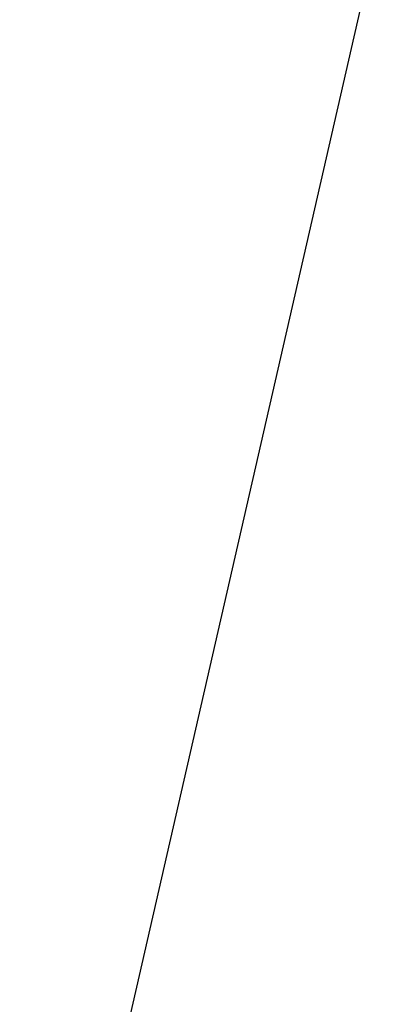
# Model space of a CAD drawing. Units: inches. Extents: x 3590 to 5167, y 65 to 1917.
# Tile 89 of 100: x 5052.4275 to 5052.5773, y 1788.6144 to 1789.0318. Entities that reach past the tile are written whole.
import ezdxf

# ---------------------------------------------------------------- set-up
doc = ezdxf.new("R2010")
doc.units = ezdxf.units.IN
for name, color, linetype, lineweight in [('A-ANNO-DIMS', 2, 'Continuous', 18), ('A-FLOR-PATT', 8, 'Continuous', 13), ('L-PLNT', 94, 'Continuous', 18)]:
    doc.layers.add(name, color=color, linetype=linetype, lineweight=lineweight)
doc.layers.add('DIENHOA', color=3, linetype='Continuous')
doc.styles.get("Standard").update_dxf_attribs({"font": 'arial.ttf'})
doc.dimstyles.new('ISO-25', dxfattribs={"dimtxt": 9, "dimasz": 2.5, "dimexe": 1.25, "dimexo": 0.625, "dimtad": 1, "dimdec": 1, "dimlunit": 3, "dimtxsty": 'Standard', "dimcen": 2.5, "dimadec": 0, "dimazin": 0, "dimtfac": 1, "dimtdec": 1, "dimtmove": 0, "dimatfit": 3, "dimfxl": 1, "dimarcsym": 0})

# ---------------------------------------------------------------- blocks, each defined once
blk = doc.blocks.new('Cay03_mb')
at = {"layer": 'DIENHOA'}
blk.add_lwpolyline([(112.868, 491.948), (95.994, 419.691), (79.461, 347.371), (63.915, 276.46), (50.006, 208.43), (38.381, 144.752), (29.688, 86.901), (24.574, 36.346), (23.687, -5.439)], dxfattribs=at)
blk = doc.blocks.new('*D323')
at = {"layer": 'A-ANNO-DIMS', "color": 0, "lineweight": -2, "transparency": 16777216}
for p, q in [((5069.17227, 1795.21603), (5069.17227, 1874.95034)), ((5065.43703, 1795.21603), (5070.42227, 1795.21603)), ((5069.17227, 1769.30924), (5069.17227, 1792.71603)), ((5065.43703, 1766.80924), (5070.42227, 1766.80924))]:
    blk.add_line(p, q, dxfattribs=at)
at = {"layer": 'A-ANNO-DIMS', "color": 0, "transparency": 16777216}
for points in [[(5068.75561, 1792.71603), (5069.58894, 1792.71603), (5069.17227, 1795.21603)], [(5068.75561, 1769.30924), (5069.58894, 1769.30924), (5069.17227, 1766.80924)]]:
    blk.add_solid(points, dxfattribs=at)
at = {"layer": 'Defpoints', "color": 0, "transparency": 16777216}
for p in [(5064.81203, 1795.21603), (5069.17227, 1795.21603), (5064.81203, 1766.80924)]:
    blk.add_point(p, dxfattribs=at)
at = {"layer": 'A-ANNO-DIMS', "color": 0, "transparency": 16777216, "insert": (5063.89379, 1836.33318), "char_height": 9, "attachment_point": 5, "rotation": 90}
blk.add_mtext('2\'-4 1/2" TYP.', dxfattribs=at)

msp = doc.modelspace()

# ---------------------------------------------------------------- hatches: boundary and pattern name
at = {"layer": 'A-FLOR-PATT', "transparency": 33554687}
h = msp.add_hatch(dxfattribs=at)
h.set_pattern_fill('AR-HBONE', color=256, scale=0.2)
h.set_pattern_definition([(45, (-588.972, 0), (0, 28.73682), [60.96, -20.32]), (135, (-574.604, 14.368), (3e-15, 28.73682), [60.96, -20.32])])
h.paths.add_polyline_path([(5071.27403, 1796.99898), (4933.27403, 1796.99898), (4933.27403, 1753.99898), (4962.77403, 1753.99898, -0.414214), (4928.77403, 1719.99898), (4933.27403, 1718.99898), (4933.27403, 1334.99898), (5071.27403, 1334.99898)])
h.paths.add_polyline_path([(4951.78002, 1521.0767), (4951.7151, 1521.0404), (4951.56345, 1520.89532)], flags=16)
h.paths.add_polyline_path([(4952.267, 1521.37645), (4952.1977, 1521.37111), (4952.19823, 1521.35558)], flags=0)
h.paths.add_polyline_path([(4967.05076, 1529.72832), (4965.23122, 1528.69444), (4963.41109, 1527.71401), (4961.75649, 1526.85081), (4963.58887, 1527.44938), (4964.03555, 1527.47802), (4962.9755, 1527.24902), (4961.76022, 1526.85203), (4959.79219, 1525.83406), (4958.00498, 1524.89483), (4956.24031, 1523.92961), (4954.50395, 1522.91854), (4954.1294, 1522.68163), (4953.36051, 1521.99688), (4953.36558, 1521.99754), (4953.605, 1522.06367), (4955.10605, 1522.76083), (4956.92108, 1523.43405), (4958.67784, 1523.91513), (4960.35834, 1524.20036), (4961.94456, 1524.28606), (4964.17144, 1524.10849), (4965.95752, 1523.30903), (4963.86273, 1522.97565), (4965.18742, 1522.49898), (4963.36614, 1522.49715), (4961.54526, 1522.48682), (4959.76359, 1522.46077), (4958.30414, 1522.4188), (4957.97356, 1522.38829), (4956.30692, 1522.2324), (4954.71821, 1522.07143), (4953.25077, 1521.89915), (4953.52509, 1521.62277), (4954.33087, 1521.37883), (4956.24263, 1521.22987), (4958.03913, 1520.92952), (4959.68424, 1520.48339), (4961.16007, 1519.89569), (4963.10699, 1518.80022), (4964.39286, 1517.32518), (4962.97306, 1517.72596), (4964.55841, 1516.66059), (4965.40664, 1515.70779), (4963.50733, 1516.32179), (4961.67995, 1517.0051), (4959.93478, 1517.74489), (4958.2821, 1518.52833), (4956.73216, 1519.34257), (4955.29527, 1520.17478), (4954.67155, 1520.57237), (4954.51279, 1520.6271), (4955.65848, 1519.31837), (4956.70263, 1517.98232), (4957.64403, 1516.64663), (4958.48545, 1515.33439), (4959.54998, 1513.52398), (4960.43768, 1511.76936), (4958.84107, 1513.6196), (4957.45175, 1515.3249), (4955.8186, 1517.45855), (4956.66537, 1515.44764), (4957.11109, 1513.92292), (4957.44681, 1511.71434), (4957.07641, 1509.79288), (4956.53757, 1511.1103), (4955.99231, 1512.56892), (4955.44448, 1514.12509), (4954.89794, 1515.73518), (4954.35653, 1517.35553), (4953.82412, 1518.94251), (4953.30455, 1520.45247), (4953.06452, 1521.11563), (4952.97143, 1521.14607), (4952.94932, 1521.08646), (4952.72981, 1520.19905), (4953.3698, 1518.02364), (4953.75708, 1516.37279), (4954.05124, 1514.76538), (4954.26449, 1513.22121), (4954.47124, 1511.13121), (4954.4971, 1510.40174), (4954.40903, 1511.76006), (4954.26449, 1513.22121), (4954.05124, 1514.76538), (4953.75708, 1516.37279), (4953.3698, 1518.02364), (4952.87718, 1519.69813), (4952.7161, 1520.1412), (4952.53301, 1519.05871), (4952.37428, 1517.78881), (4952.21925, 1516.31167), (4952.04598, 1514.59986), (4951.83253, 1512.62598), (4951.55697, 1510.36259), (4951.20331, 1512.16818), (4950.85168, 1514.33931), (4950.98529, 1516.37594), (4951.6596, 1518.28625), (4952.59261, 1520.48085), (4952.35664, 1521.1299), (4951.85502, 1520.32753), (4950.83901, 1518.90828), (4949.77675, 1517.58658), (4948.91554, 1516.61731), (4948.11099, 1515.2561), (4947.0891, 1513.55389), (4945.88937, 1511.61495), (4946.32587, 1513.40232), (4946.5624, 1514.24913), (4945.52771, 1513.32668), (4944.58105, 1512.53126), (4946.01774, 1514.50825), (4947.2044, 1516.04763), (4947.89331, 1517.31331), (4949.30686, 1518.76446), (4950.41417, 1519.76716), (4950.45131, 1519.80628), (4952.267, 1521.37645), (4951.64457, 1521.49317), (4950.40371, 1521.17954), (4948.04447, 1520.35868), (4946.11863, 1519.45198), (4944.57182, 1518.47484), (4943.34962, 1517.44265), (4941.99695, 1515.91971), (4941.66146, 1515.27475), (4942.81332, 1516.98973), (4944.57182, 1518.47484), (4946.11863, 1519.45198), (4948.04447, 1520.35868), (4950.40371, 1521.17954), (4951.64457, 1521.49317), (4949.64678, 1521.86781), (4948.59979, 1521.75633), (4947.12629, 1521.5699), (4945.42015, 1521.34763), (4943.44969, 1521.10462), (4941.18319, 1520.85596), (4942.86028, 1521.61265), (4943.87308, 1522.03014), (4942.95216, 1521.9093), (4941.40968, 1521.48512), (4939.54287, 1520.67019), (4938.96775, 1520.2255), (4940.73284, 1521.29899), (4942.95216, 1521.9093), (4943.70184, 1522.00767), (4945.89419, 1522.69998), (4947.56488, 1522.71399), (4948.92086, 1522.56573), (4951.13144, 1522.18271), (4950.97062, 1522.2969), (4948.12924, 1523.00563), (4946.03496, 1523.70671), (4944.23235, 1524.52143), (4942.70692, 1525.46111), (4941.44419, 1526.53707), (4940.42968, 1527.76062), (4939.6489, 1529.14306), (4941.42091, 1528.12232), (4943.14742, 1527.13248), (4944.84093, 1526.17457), (4946.51394, 1525.24959), (4948.17893, 1524.35855), (4948.36457, 1524.26336), (4946.47531, 1526.04459), (4945.18083, 1527.54042), (4944.19039, 1529.03339), (4943.49559, 1530.53985), (4943.27808, 1531.3597), (4942.49849, 1531.91903), (4943.11353, 1531.76249), (4942.95927, 1533.6586), (4944.13953, 1531.9886), (4944.61171, 1531.32339), (4946.20163, 1530.46341), (4947.48567, 1529.50925), (4948.79027, 1528.22649), (4950.36754, 1526.23746), (4949.48547, 1528.15549), (4948.85128, 1530.12254), (4948.49054, 1532.04127), (4948.38105, 1533.91822), (4948.50062, 1535.7599), (4948.82704, 1537.57284), (4949.41803, 1535.56526), (4949.95684, 1533.56932), (4950.46414, 1531.5861), (4950.96058, 1529.6167), (4951.3911, 1527.95448), (4951.72352, 1530.68689), (4952.20106, 1532.57994), (4952.88914, 1534.32964), (4953.77035, 1535.95123), (4954.82726, 1537.45995), (4954.52145, 1535.38966), (4954.27314, 1533.93684), (4955.57999, 1535.6627), (4956.74758, 1536.73859), (4956.15852, 1534.78029), (4955.58917, 1532.87334), (4955.04336, 1531.00581), (4954.52493, 1529.16576), (4954.03771, 1527.34127), (4953.63833, 1525.73298), (4953.61143, 1525.58564), (4953.39805, 1524.16565), (4953.38219, 1524.00887), (4954.06955, 1525.47563), (4954.91212, 1527.02173), (4956.13627, 1528.89351), (4957.84668, 1530.57701), (4959.37601, 1531.54014), (4958.25596, 1530.10398), (4957.14284, 1528.66291), (4956.06626, 1527.24305), (4955.05579, 1525.87054), (4954.14104, 1524.57149), (4953.35159, 1523.37204), (4953.31079, 1523.30299), (4953.27253, 1522.92478), (4953.26102, 1522.38213), (4954.1031, 1523.37273), (4954.63005, 1524.28376), (4955.96149, 1526.35767), (4957.23002, 1528.12969), (4958.42057, 1529.60864), (4960.03671, 1531.36792), (4961.3736, 1532.3752), (4962.1015, 1532.77), (4961.06994, 1531.06113), (4959.98733, 1529.43811), (4958.86851, 1527.90803), (4958.15046, 1527.00742), (4959.80291, 1528.00314), (4961.58854, 1528.79257), (4963.39087, 1529.32783), (4965.21118, 1529.63205)], flags=16)
h.paths.add_polyline_path([(4962.94387, 1523.18187), (4961.10714, 1523.42192), (4960.39205, 1523.36158), (4962.34964, 1523.33061)], flags=0)
h.paths.add_polyline_path([(5049.54129, 1584.55089), (5049.47636, 1584.51458), (5049.32471, 1584.3695)], flags=16)
h.paths.add_polyline_path([(5050.02827, 1584.85063), (5049.95897, 1584.84529), (5049.95949, 1584.82976)], flags=0)
h.paths.add_polyline_path([(5042.33308, 1581.94902), (5043.8799, 1582.92616), (5045.80573, 1583.83286), (5048.16498, 1584.65372), (5049.40583, 1584.96736), (5047.40804, 1585.34199), (5046.36106, 1585.23052), (5044.88755, 1585.04408), (5043.18142, 1584.82181), (5041.21095, 1584.5788), (5038.94446, 1584.33014), (5040.62155, 1585.08683), (5041.63434, 1585.50432), (5040.71343, 1585.38348), (5039.17095, 1584.9593), (5037.30414, 1584.14438), (5036.72901, 1583.69969), (5038.4941, 1584.77317), (5040.71343, 1585.38348), (5041.4631, 1585.48185), (5043.65545, 1586.17416), (5045.32615, 1586.18818), (5046.68212, 1586.03992), (5048.8927, 1585.6569), (5048.73188, 1585.77108), (5045.89051, 1586.47981), (5043.79622, 1587.18089), (5041.99361, 1587.99561), (5040.46818, 1588.9353), (5039.20546, 1590.01125), (5038.19095, 1591.2348), (5037.41016, 1592.61725), (5039.18217, 1591.5965), (5040.90868, 1590.60667), (5042.6022, 1589.64876), (5044.2752, 1588.72378), (5045.94019, 1587.83274), (5046.12584, 1587.73754), (5044.23658, 1589.51878), (5042.9421, 1591.01461), (5041.95166, 1592.50757), (5041.25685, 1594.01403), (5041.03935, 1594.83388), (5040.25976, 1595.39321), (5040.8748, 1595.23667), (5040.72054, 1597.13279), (5041.9008, 1595.46278), (5042.37297, 1594.79758), (5043.96289, 1593.93759), (5045.24694, 1592.98344), (5046.55153, 1591.70068), (5048.12881, 1589.71164), (5047.24673, 1591.62967), (5046.61254, 1593.59672), (5046.2518, 1595.51546), (5046.14232, 1597.3924), (5046.26189, 1599.23408), (5046.5883, 1601.04703), (5047.17929, 1599.03944), (5047.71811, 1597.0435), (5048.22541, 1595.06028), (5048.72184, 1593.09089), (5049.15237, 1591.42866), (5049.48478, 1594.16107), (5049.96233, 1596.05412), (5050.65041, 1597.80382), (5051.53161, 1599.42541), (5052.58852, 1600.93414), (5052.28271, 1598.86384), (5052.03441, 1597.41102), (5053.34126, 1599.13689), (5054.50884, 1600.21277), (5053.91979, 1598.25447), (5053.35044, 1596.34752), (5052.80463, 1594.47999), (5052.2862, 1592.63995), (5051.79898, 1590.81546), (5051.39959, 1589.20716), (5051.3727, 1589.05983), (5051.15931, 1587.63984), (5051.14346, 1587.48305), (5051.83082, 1588.94982), (5052.67339, 1590.49592), (5053.89754, 1592.3677), (5055.60794, 1594.05119), (5057.13728, 1595.01432), (5056.01722, 1593.57817), (5054.90411, 1592.1371), (5053.82752, 1590.71724), (5052.81705, 1589.34472), (5051.9023, 1588.04567), (5051.11286, 1586.84622), (5051.07205, 1586.77718), (5051.03379, 1586.39896), (5051.02228, 1585.85631), (5051.86437, 1586.84692), (5052.39131, 1587.75794), (5053.72275, 1589.83185), (5054.99128, 1591.60387), (5056.18183, 1593.08282), (5057.79798, 1594.84211), (5059.13486, 1595.84938), (5059.86276, 1596.24419), (5058.83121, 1594.53531), (5057.7486, 1592.9123), (5056.62978, 1591.38221), (5055.91173, 1590.4816), (5057.56418, 1591.47732), (5059.34981, 1592.26675), (5061.15214, 1592.80202), (5062.97245, 1593.10624), (5064.81203, 1593.20251), (5062.99248, 1592.16863), (5061.17235, 1591.18819), (5059.51775, 1590.325), (5061.35014, 1590.92356), (5061.79682, 1590.95221), (5060.73676, 1590.7232), (5059.52148, 1590.32622), (5057.55345, 1589.30825), (5055.76625, 1588.36901), (5054.00157, 1587.40379), (5052.26521, 1586.39273), (5051.89067, 1586.15581), (5051.12177, 1585.47106), (5051.12684, 1585.47172), (5051.36627, 1585.53786), (5052.86732, 1586.23502), (5054.68234, 1586.90824), (5056.4391, 1587.38931), (5058.1196, 1587.67454), (5059.70582, 1587.76024), (5061.93271, 1587.58268), (5063.71878, 1586.78321), (5061.62399, 1586.44983), (5062.94869, 1585.97317), (5061.12741, 1585.97133), (5059.30653, 1585.961), (5057.52486, 1585.93496), (5056.06541, 1585.89299), (5055.73482, 1585.86247), (5054.06819, 1585.70658), (5052.47947, 1585.54561), (5051.01204, 1585.37333), (5051.28635, 1585.09695), (5052.09214, 1584.85301), (5054.00389, 1584.70406), (5055.8004, 1584.4037), (5057.44551, 1583.95757), (5058.92133, 1583.36987), (5060.86825, 1582.27441), (5062.15413, 1580.79937), (5060.73433, 1581.20015), (5062.31967, 1580.13477), (5063.1679, 1579.18198), (5061.2686, 1579.79597), (5059.44122, 1580.47928), (5057.69605, 1581.21908), (5056.04336, 1582.00251), (5054.49343, 1582.81675), (5053.05653, 1583.64897), (5052.43281, 1584.04656), (5052.27405, 1584.10128), (5053.41974, 1582.79255), (5054.4639, 1581.4565), (5055.40529, 1580.12081), (5056.24672, 1578.80858), (5057.31125, 1576.99816), (5058.19895, 1575.24354), (5056.60234, 1577.09378), (5055.21301, 1578.79908), (5053.57987, 1580.93274), (5054.42664, 1578.92183), (5054.87235, 1577.3971), (5055.20808, 1575.18852), (5054.83767, 1573.26706), (5054.29883, 1574.58448), (5053.75357, 1576.0431), (5053.20575, 1577.59927), (5052.6592, 1579.20936), (5052.1178, 1580.82971), (5051.58538, 1582.41669), (5051.06582, 1583.92666), (5050.82578, 1584.58981), (5050.7327, 1584.62025), (5050.71058, 1584.56064), (5050.49108, 1583.67323), (5051.13107, 1581.49782), (5051.51835, 1579.84698), (5051.8125, 1578.23957), (5052.02575, 1576.69539), (5052.23251, 1574.6054), (5052.25836, 1573.87593), (5052.1703, 1575.23424), (5052.02575, 1576.69539), (5051.8125, 1578.23957), (5051.51835, 1579.84698), (5051.13107, 1581.49782), (5050.63844, 1583.17231), (5050.47736, 1583.61538), (5050.29428, 1582.53289), (5050.13554, 1581.26299), (5049.98051, 1579.78585), (5049.80724, 1578.07405), (5049.59379, 1576.10016), (5049.31823, 1573.83678), (5048.96458, 1575.64237), (5048.61294, 1577.8135), (5048.74656, 1579.85012), (5049.42086, 1581.76043), (5050.35388, 1583.95503), (5050.1179, 1584.60408), (5049.61629, 1583.80172), (5048.60027, 1582.38246), (5047.53801, 1581.06076), (5046.67681, 1580.09149), (5045.87225, 1578.73029), (5044.85036, 1577.02808), (5043.65063, 1575.08913), (5044.08713, 1576.8765), (5044.32366, 1577.72331), (5043.28898, 1576.80086), (5042.34232, 1576.00545), (5043.779, 1577.98243), (5044.96566, 1579.52182), (5045.65457, 1580.78749), (5047.06813, 1582.23865), (5048.17543, 1583.24134), (5048.21258, 1583.28047), (5050.02827, 1584.85063), (5049.40583, 1584.96736), (5048.16498, 1584.65372), (5045.80573, 1583.83286), (5043.8799, 1582.92616), (5042.33308, 1581.94902), (5041.11088, 1580.91684), (5039.75821, 1579.39389), (5039.42272, 1578.74894), (5040.57458, 1580.46391)], flags=16)
h.paths.add_polyline_path([(4954.79872, 1533.12029), (4954.26249, 1532.07935), (4953.83112, 1530.93464), (4953.50472, 1529.63602), (4953.28338, 1528.13331), (4953.16721, 1526.37637), (4953.15631, 1524.31504), (4953.27669, 1521.23629), (4952.80168, 1521.84177), (4951.55695, 1521.99789), (4950.97575, 1521.9613), (4952.66059, 1521.94097), (4952.80168, 1521.84177), (4953.15249, 1523.59258), (4953.16721, 1526.37637), (4953.28338, 1528.13331), (4953.60929, 1530.34598), (4954.45558, 1532.59174)], flags=0)
h.paths.add_polyline_path([(5050.56294, 1585.31596), (5049.31822, 1585.47208), (5048.73702, 1585.43548), (5050.42186, 1585.41516), (5050.56294, 1585.31596), (5050.91375, 1587.06676), (5050.92848, 1589.85056), (5051.04465, 1591.6075), (5051.37055, 1593.82017), (5052.21684, 1596.06593), (5052.55999, 1596.59447), (5052.02375, 1595.55353), (5051.59238, 1594.40883), (5051.26598, 1593.1102), (5051.04465, 1591.6075), (5050.92848, 1589.85056), (5050.91757, 1587.78922), (5051.03795, 1584.71048)], flags=0)
h.paths.add_polyline_path([(5058.15332, 1586.83576), (5060.11091, 1586.80479), (5060.70514, 1586.65605), (5058.8684, 1586.8961)], flags=0)
h.paths.add_polyline_path([(5049.54129, 1430.93611), (5049.47636, 1430.8998), (5049.32471, 1430.75472)], flags=16)
h.paths.add_polyline_path([(5050.02827, 1431.23585), (5049.95897, 1431.23051), (5049.95949, 1431.21498)], flags=0)
h.paths.add_polyline_path([(5046.5883, 1447.43225), (5047.17929, 1445.42467), (5047.71811, 1443.42872), (5048.22541, 1441.4455), (5048.72184, 1439.47611), (5049.15237, 1437.81388), (5049.48478, 1440.5463), (5049.96233, 1442.43934), (5050.65041, 1444.18904), (5051.53161, 1445.81063), (5052.58852, 1447.31936), (5052.28271, 1445.24906), (5052.03441, 1443.79624), (5053.34126, 1445.52211), (5054.50884, 1446.59799), (5053.91979, 1444.63969), (5053.35044, 1442.73274), (5052.80463, 1440.86521), (5052.2862, 1439.02517), (5051.79898, 1437.20068), (5051.39959, 1435.59238), (5051.3727, 1435.44505), (5051.15931, 1434.02506), (5051.14346, 1433.86828), (5051.83082, 1435.33504), (5052.67339, 1436.88114), (5053.89754, 1438.75292), (5055.60794, 1440.43641), (5057.13728, 1441.39954), (5056.01722, 1439.96339), (5054.90411, 1438.52232), (5053.82752, 1437.10246), (5052.81705, 1435.72994), (5051.9023, 1434.4309), (5051.11286, 1433.23145), (5051.07205, 1433.1624), (5051.03379, 1432.78418), (5051.02228, 1432.24153), (5051.86437, 1433.23214), (5052.39131, 1434.14316), (5053.72275, 1436.21707), (5054.99128, 1437.98909), (5056.18183, 1439.46805), (5057.79798, 1441.22733), (5059.13486, 1442.23461), (5059.86276, 1442.62941), (5058.83121, 1440.92053), (5057.7486, 1439.29752), (5056.62978, 1437.76743), (5055.91173, 1436.86682), (5057.56418, 1437.86255), (5059.34981, 1438.65197), (5061.15214, 1439.18724), (5062.97245, 1439.49146), (5064.81203, 1439.58773), (5062.99248, 1438.55385), (5061.17235, 1437.57342), (5059.51775, 1436.71022), (5061.35014, 1437.30879), (5061.79682, 1437.33743), (5060.73676, 1437.10842), (5059.52148, 1436.71144), (5057.55345, 1435.69347), (5055.76625, 1434.75423), (5054.00157, 1433.78901), (5052.26521, 1432.77795), (5051.89067, 1432.54103), (5051.12177, 1431.85628), (5051.12684, 1431.85694), (5051.36627, 1431.92308), (5052.86732, 1432.62024), (5054.68234, 1433.29346), (5056.4391, 1433.77453), (5058.1196, 1434.05976), (5059.70582, 1434.14546), (5061.93271, 1433.9679), (5063.71878, 1433.16843), (5061.62399, 1432.83505), (5062.94869, 1432.35839), (5061.12741, 1432.35655), (5059.30653, 1432.34623), (5057.52486, 1432.32018), (5056.06541, 1432.27821), (5055.73482, 1432.24769), (5054.06819, 1432.09181), (5052.47947, 1431.93083), (5051.01204, 1431.75856), (5051.28635, 1431.48218), (5052.09214, 1431.23823), (5054.00389, 1431.08928), (5055.8004, 1430.78892), (5057.44551, 1430.34279), (5058.92133, 1429.75509), (5060.86825, 1428.65963), (5062.15413, 1427.18459), (5060.73433, 1427.58537), (5062.31967, 1426.52), (5063.1679, 1425.5672), (5061.2686, 1426.18119), (5059.44122, 1426.86451), (5057.69605, 1427.6043), (5056.04336, 1428.38773), (5054.49343, 1429.20197), (5053.05653, 1430.03419), (5052.43281, 1430.43178), (5052.27405, 1430.48651), (5053.41974, 1429.17777), (5054.4639, 1427.84172), (5055.40529, 1426.50603), (5056.24672, 1425.1938), (5057.31125, 1423.38338), (5058.19895, 1421.62877), (5056.60234, 1423.479), (5055.21301, 1425.1843), (5053.57987, 1427.31796), (5054.42664, 1425.30705), (5054.87235, 1423.78233), (5055.20808, 1421.57374), (5054.83767, 1419.65228), (5054.29883, 1420.9697), (5053.75357, 1422.42832), (5053.20575, 1423.9845), (5052.6592, 1425.59458), (5052.1178, 1427.21493), (5051.58538, 1428.80191), (5051.06582, 1430.31188), (5050.82578, 1430.97503), (5050.7327, 1431.00547), (5050.71058, 1430.94586), (5050.49108, 1430.05845), (5051.13107, 1427.88305), (5051.51835, 1426.2322), (5051.8125, 1424.62479), (5052.02575, 1423.08061), (5052.23251, 1420.99062), (5052.25836, 1420.26115), (5052.1703, 1421.61947), (5052.02575, 1423.08061), (5051.8125, 1424.62479), (5051.51835, 1426.2322), (5051.13107, 1427.88305), (5050.63844, 1429.55753), (5050.47736, 1430.0006), (5050.29428, 1428.91811), (5050.13554, 1427.64821), (5049.98051, 1426.17107), (5049.80724, 1424.45927), (5049.59379, 1422.48539), (5049.31823, 1420.222), (5048.96458, 1422.02759), (5048.61294, 1424.19872), (5048.74656, 1426.23534), (5049.42086, 1428.14565), (5050.35388, 1430.34025), (5050.1179, 1430.98931), (5049.61629, 1430.18694), (5048.60027, 1428.76768), (5047.53801, 1427.44598), (5046.67681, 1426.47671), (5045.87225, 1425.11551), (5044.85036, 1423.4133), (5043.65063, 1421.47435), (5044.08713, 1423.26172), (5044.32366, 1424.10854), (5043.28898, 1423.18608), (5042.34232, 1422.39067), (5043.779, 1424.36765), (5044.96566, 1425.90704), (5045.65457, 1427.17272), (5047.06813, 1428.62387), (5048.17543, 1429.62657), (5048.21258, 1429.66569), (5050.02827, 1431.23585), (5049.40583, 1431.35258), (5048.16498, 1431.03894), (5045.80573, 1430.21809), (5043.8799, 1429.31139), (5042.33308, 1428.33424), (5041.11088, 1427.30206), (5039.75821, 1425.77911), (5039.42272, 1425.13416), (5040.57458, 1426.84914), (5042.33308, 1428.33424), (5043.8799, 1429.31139), (5045.80573, 1430.21809), (5048.16498, 1431.03894), (5049.40583, 1431.35258), (5047.40804, 1431.72722), (5046.36106, 1431.61574), (5044.88755, 1431.42931), (5043.18142, 1431.20704), (5041.21095, 1430.96402), (5038.94446, 1430.71536), (5040.62155, 1431.47205), (5041.63434, 1431.88954), (5040.71343, 1431.76871), (5039.17095, 1431.34453), (5037.30414, 1430.5296), (5036.72901, 1430.08491), (5038.4941, 1431.1584), (5040.71343, 1431.76871), (5041.4631, 1431.86707), (5043.65545, 1432.55939), (5045.32615, 1432.5734), (5046.68212, 1432.42514), (5048.8927, 1432.04212), (5048.73188, 1432.1563), (5045.89051, 1432.86503), (5043.79622, 1433.56611), (5041.99361, 1434.38083), (5040.46818, 1435.32052), (5039.20546, 1436.39648), (5038.19095, 1437.62002), (5037.41016, 1439.00247), (5039.18217, 1437.98172), (5040.90868, 1436.99189), (5042.6022, 1436.03398), (5044.2752, 1435.109), (5045.94019, 1434.21796), (5046.12584, 1434.12276), (5044.23658, 1435.904), (5042.9421, 1437.39983), (5041.95166, 1438.8928), (5041.25685, 1440.39925), (5041.03935, 1441.2191), (5040.25976, 1441.77844), (5040.8748, 1441.62189), (5040.72054, 1443.51801), (5041.9008, 1441.848), (5042.37297, 1441.1828), (5043.96289, 1440.32282), (5045.24694, 1439.36866), (5046.55153, 1438.0859), (5048.12881, 1436.09686), (5047.24673, 1438.01489), (5046.61254, 1439.98195), (5046.2518, 1441.90068), (5046.14232, 1443.77762), (5046.26189, 1445.6193)], flags=16)
h.paths.add_polyline_path([(5052.38176, 1444.25496), (5051.62263, 1442.77987), (5052.02375, 1441.93875), (5052.55999, 1442.9797)], flags=0)
h.paths.add_polyline_path([(5050.56294, 1431.70118), (5049.31822, 1431.8573), (5048.73702, 1431.82071), (5050.42186, 1431.80038)], flags=0)
h.paths.add_polyline_path([(5058.15332, 1433.22098), (5060.11091, 1433.19001), (5060.70514, 1433.04127), (5058.8684, 1433.28132)], flags=0)
h.paths.add_polyline_path([(5049.54129, 1352.28535), (5049.47636, 1352.24904), (5049.32471, 1352.10396)], flags=16)
h.paths.add_polyline_path([(5050.02827, 1352.58509), (5049.95897, 1352.57975), (5049.95949, 1352.56422)], flags=0)
h.paths.add_polyline_path([(5046.5883, 1368.78149), (5047.17929, 1366.7739), (5047.71811, 1364.77796), (5048.22541, 1362.79474), (5048.72184, 1360.82534), (5049.15237, 1359.16312), (5049.48478, 1361.89553), (5049.96233, 1363.78858), (5050.65041, 1365.53828), (5051.53161, 1367.15987), (5052.58852, 1368.6686), (5052.28271, 1366.5983), (5052.03441, 1365.14548), (5053.34126, 1366.87135), (5054.50884, 1367.94723), (5053.91979, 1365.98893), (5053.35044, 1364.08198), (5052.80463, 1362.21445), (5052.2862, 1360.37441), (5051.79898, 1358.54992), (5051.39959, 1356.94162), (5051.3727, 1356.79428), (5051.15931, 1355.37429), (5051.14346, 1355.21751), (5051.83082, 1356.68428), (5052.67339, 1358.23037), (5053.89754, 1360.10216), (5055.60794, 1361.78565), (5057.13728, 1362.74878), (5056.01722, 1361.31262), (5054.90411, 1359.87155), (5053.82752, 1358.4517), (5052.81705, 1357.07918), (5051.9023, 1355.78013), (5051.11286, 1354.58068), (5051.07205, 1354.51164), (5051.03379, 1354.13342), (5051.02228, 1353.59077), (5051.86437, 1354.58137), (5052.39131, 1355.4924), (5053.72275, 1357.56631), (5054.99128, 1359.33833), (5056.18183, 1360.81728), (5057.79798, 1362.57656), (5059.13486, 1363.58384), (5059.86276, 1363.97864), (5058.83121, 1362.26977), (5057.7486, 1360.64675), (5056.62978, 1359.11667), (5055.91173, 1358.21606), (5057.56418, 1359.21178), (5059.34981, 1360.00121), (5061.15214, 1360.53648), (5062.97245, 1360.84069), (5064.81203, 1360.93697), (5062.99248, 1359.90308), (5061.17235, 1358.92265), (5059.51775, 1358.05946), (5061.35014, 1358.65802), (5061.79682, 1358.68666), (5060.73676, 1358.45766), (5059.52148, 1358.06068), (5057.55345, 1357.0427), (5055.76625, 1356.10347), (5054.00157, 1355.13825), (5052.26521, 1354.12718), (5051.89067, 1353.89027), (5051.12177, 1353.20552), (5051.12684, 1353.20618), (5051.36627, 1353.27231), (5052.86732, 1353.96947), (5054.68234, 1354.6427), (5056.4391, 1355.12377), (5058.1196, 1355.409), (5059.70582, 1355.4947), (5061.93271, 1355.31713), (5063.71878, 1354.51767), (5061.62399, 1354.18429), (5062.94869, 1353.70763), (5061.12741, 1353.70579), (5059.30653, 1353.69546), (5057.52486, 1353.66942), (5056.06541, 1353.62744), (5055.73482, 1353.59693), (5054.06819, 1353.44104), (5052.47947, 1353.28007), (5051.01204, 1353.10779), (5051.28635, 1352.83141), (5052.09214, 1352.58747), (5054.00389, 1352.43852), (5055.8004, 1352.13816), (5057.44551, 1351.69203), (5058.92133, 1351.10433), (5060.86825, 1350.00887), (5062.15413, 1348.53382), (5060.73433, 1348.9346), (5062.31967, 1347.86923), (5063.1679, 1346.91643), (5061.2686, 1347.53043), (5059.44122, 1348.21374), (5057.69605, 1348.95353), (5056.04336, 1349.73697), (5054.49343, 1350.55121), (5053.05653, 1351.38342), (5052.43281, 1351.78101), (5052.27405, 1351.83574), (5053.41974, 1350.52701), (5054.4639, 1349.19096), (5055.40529, 1347.85527), (5056.24672, 1346.54303), (5057.31125, 1344.73262), (5058.19895, 1342.978), (5056.60234, 1344.82824), (5055.21301, 1346.53354), (5053.57987, 1348.6672), (5054.42664, 1346.65629), (5054.87235, 1345.13156), (5055.20808, 1342.92298), (5054.83767, 1341.00152), (5054.29883, 1342.31894), (5053.75357, 1343.77756), (5053.20575, 1345.33373), (5052.6592, 1346.94382), (5052.1178, 1348.56417), (5051.58538, 1350.15115), (5051.06582, 1351.66111), (5050.82578, 1352.32427), (5050.7327, 1352.35471), (5050.71058, 1352.2951), (5050.49108, 1351.40769), (5051.13107, 1349.23228), (5051.51835, 1347.58144), (5051.8125, 1345.97403), (5052.02575, 1344.42985), (5052.23251, 1342.33986), (5052.25836, 1341.61039), (5052.1703, 1342.9687), (5052.02575, 1344.42985), (5051.8125, 1345.97403), (5051.51835, 1347.58144), (5051.13107, 1349.23228), (5050.63844, 1350.90677), (5050.47736, 1351.34984), (5050.29428, 1350.26735), (5050.13554, 1348.99745), (5049.98051, 1347.52031), (5049.80724, 1345.80851), (5049.59379, 1343.83462), (5049.31823, 1341.57124), (5048.96458, 1343.37683), (5048.61294, 1345.54796), (5048.74656, 1347.58458), (5049.42086, 1349.49489), (5050.35388, 1351.68949), (5050.1179, 1352.33854), (5049.61629, 1351.53617), (5048.60027, 1350.11692), (5047.53801, 1348.79522), (5046.67681, 1347.82595), (5045.87225, 1346.46475), (5044.85036, 1344.76253), (5043.65063, 1342.82359), (5044.08713, 1344.61096), (5044.32366, 1345.45777), (5043.28898, 1344.53532), (5042.34232, 1343.7399), (5043.779, 1345.71689), (5044.96566, 1347.25627), (5045.65457, 1348.52195), (5047.06813, 1349.9731), (5048.17543, 1350.9758), (5048.21258, 1351.01493), (5050.02827, 1352.58509), (5049.40583, 1352.70181), (5048.16498, 1352.38818), (5045.80573, 1351.56732), (5043.8799, 1350.66062), (5042.33308, 1349.68348), (5041.11088, 1348.65129), (5039.75821, 1347.12835), (5039.42272, 1346.4834), (5040.57458, 1348.19837), (5042.33308, 1349.68348), (5043.8799, 1350.66062), (5045.80573, 1351.56732), (5048.16498, 1352.38818), (5049.40583, 1352.70181), (5047.40804, 1353.07645), (5046.36106, 1352.96498), (5044.88755, 1352.77854), (5043.18142, 1352.55627), (5041.21095, 1352.31326), (5038.94446, 1352.0646), (5040.62155, 1352.82129), (5041.63434, 1353.23878), (5040.71343, 1353.11794), (5039.17095, 1352.69376), (5037.30414, 1351.87884), (5036.72901, 1351.43415), (5038.4941, 1352.50763), (5040.71343, 1353.11794), (5041.4631, 1353.21631), (5043.65545, 1353.90862), (5045.32615, 1353.92263), (5046.68212, 1353.77438), (5048.8927, 1353.39136), (5048.73188, 1353.50554), (5045.89051, 1354.21427), (5043.79622, 1354.91535), (5041.99361, 1355.73007), (5040.46818, 1356.66975), (5039.20546, 1357.74571), (5038.19095, 1358.96926), (5037.41016, 1360.35171), (5039.18217, 1359.33096), (5040.90868, 1358.34112), (5042.6022, 1357.38321), (5044.2752, 1356.45824), (5045.94019, 1355.5672), (5046.12584, 1355.472), (5044.23658, 1357.25323), (5042.9421, 1358.74906), (5041.95166, 1360.24203), (5041.25685, 1361.74849), (5041.03935, 1362.56834), (5040.25976, 1363.12767), (5040.8748, 1362.97113), (5040.72054, 1364.86725), (5041.9008, 1363.19724), (5042.37297, 1362.53203), (5043.96289, 1361.67205), (5045.24694, 1360.7179), (5046.55153, 1359.43513), (5048.12881, 1357.4461), (5047.24673, 1359.36413), (5046.61254, 1361.33118), (5046.2518, 1363.24992), (5046.14232, 1365.12686), (5046.26189, 1366.96854)], flags=16)
h.paths.add_polyline_path([(5052.38176, 1365.6042), (5051.62263, 1364.12911), (5052.02375, 1363.28799), (5052.55999, 1364.32893)], flags=0)
h.paths.add_polyline_path([(4951.78002, 1698.04081), (4951.7151, 1698.0045), (4951.56345, 1697.85942)], flags=16)
h.paths.add_polyline_path([(4952.267, 1698.34055), (4952.1977, 1698.33521), (4952.19823, 1698.31968)], flags=0)
h.paths.add_polyline_path([(4957.07641, 1686.75698), (4956.53757, 1688.0744), (4955.99231, 1689.53302), (4955.44448, 1691.08919), (4954.89794, 1692.69928), (4954.35653, 1694.31963), (4953.82412, 1695.90661), (4953.30455, 1697.41658), (4953.06452, 1698.07973), (4952.97143, 1698.11017), (4952.94932, 1698.05056), (4952.72981, 1697.16315), (4953.3698, 1694.98774), (4953.75708, 1693.3369), (4954.05124, 1691.72949), (4954.26449, 1690.18531), (4954.47124, 1688.09532), (4954.4971, 1687.36585), (4954.40903, 1688.72416), (4954.26449, 1690.18531), (4954.05124, 1691.72949), (4953.75708, 1693.3369), (4953.3698, 1694.98774), (4952.87718, 1696.66223), (4952.7161, 1697.1053), (4952.53301, 1696.02281), (4952.37428, 1694.75291), (4952.21925, 1693.27577), (4952.04598, 1691.56397), (4951.83253, 1689.59008), (4951.55697, 1687.3267), (4951.20331, 1689.13229), (4950.85168, 1691.30342), (4950.98529, 1693.34004), (4951.6596, 1695.25035), (4952.59261, 1697.44495), (4952.35664, 1698.09401), (4951.85502, 1697.29164), (4950.83901, 1695.87238), (4949.77675, 1694.55068), (4948.91554, 1693.58141), (4948.11099, 1692.22021), (4947.0891, 1690.518), (4945.88937, 1688.57905), (4946.32587, 1690.36642), (4946.5624, 1691.21323), (4945.52771, 1690.29078), (4944.58105, 1689.49537), (4946.01774, 1691.47235), (4947.2044, 1693.01174), (4947.89331, 1694.27741), (4949.30686, 1695.72857), (4950.41417, 1696.73127), (4950.45131, 1696.77039), (4952.267, 1698.34055), (4951.64457, 1698.45728), (4950.40371, 1698.14364), (4948.04447, 1697.32278), (4946.11863, 1696.41608), (4944.57182, 1695.43894), (4943.34962, 1694.40676), (4941.99695, 1692.88381), (4941.66146, 1692.23886), (4942.81332, 1693.95383), (4944.57182, 1695.43894), (4946.11863, 1696.41608), (4948.04447, 1697.32278), (4950.40371, 1698.14364), (4951.64457, 1698.45728), (4949.64678, 1698.83191), (4948.59979, 1698.72044), (4947.12629, 1698.53401), (4945.42015, 1698.31174), (4943.44969, 1698.06872), (4941.18319, 1697.82006), (4942.86028, 1698.57675), (4943.87308, 1698.99424), (4942.95216, 1698.8734), (4941.40968, 1698.44922), (4939.54287, 1697.6343), (4938.96775, 1697.18961), (4940.73284, 1698.26309), (4942.95216, 1698.8734), (4943.70184, 1698.97177), (4945.89419, 1699.66409), (4947.56488, 1699.6781), (4948.92086, 1699.52984), (4951.13144, 1699.14682), (4950.97062, 1699.261), (4948.12924, 1699.96973), (4946.03496, 1700.67081), (4944.23235, 1701.48553), (4942.70692, 1702.42522), (4941.44419, 1703.50117), (4940.42968, 1704.72472), (4939.6489, 1706.10717), (4941.42091, 1705.08642), (4943.14742, 1704.09659), (4944.84093, 1703.13868), (4946.51394, 1702.2137), (4948.17893, 1701.32266), (4948.36457, 1701.22746), (4946.47531, 1703.0087), (4945.18083, 1704.50453), (4944.19039, 1705.9975), (4943.49559, 1707.50395), (4943.27808, 1708.3238), (4942.49849, 1708.88314), (4943.11353, 1708.72659), (4942.95927, 1710.62271), (4944.13953, 1708.9527), (4944.61171, 1708.2875), (4946.20163, 1707.42751), (4947.48567, 1706.47336), (4948.79027, 1705.1906), (4950.36754, 1703.20156), (4949.48547, 1705.11959), (4948.85128, 1707.08664), (4948.49054, 1709.00538), (4948.38105, 1710.88232), (4948.50062, 1712.724), (4948.82704, 1714.53695), (4949.41803, 1712.52937), (4949.95684, 1710.53342), (4950.46414, 1708.5502), (4950.96058, 1706.58081), (4951.3911, 1704.91858), (4951.72352, 1707.65099), (4952.20106, 1709.54404), (4952.88914, 1711.29374), (4953.77035, 1712.91533), (4954.82726, 1714.42406), (4954.52145, 1712.35376), (4954.27314, 1710.90094), (4955.57999, 1712.62681), (4956.74758, 1713.70269), (4956.15852, 1711.74439), (4955.58917, 1709.83744), (4955.04336, 1707.96991), (4954.52493, 1706.12987), (4954.03771, 1704.30538), (4953.63833, 1702.69708), (4953.61143, 1702.54975), (4953.39805, 1701.12976), (4953.38219, 1700.97297), (4954.06955, 1702.43974), (4954.91212, 1703.98584), (4956.13627, 1705.85762), (4957.84668, 1707.54111), (4959.37601, 1708.50424), (4958.25596, 1707.06809), (4957.14284, 1705.62702), (4956.06626, 1704.20716), (4955.05579, 1702.83464), (4954.14104, 1701.53559), (4953.35159, 1700.33614), (4953.31079, 1700.2671), (4953.27253, 1699.88888), (4953.26102, 1699.34623), (4954.1031, 1700.33684), (4954.63005, 1701.24786), (4955.96149, 1703.32177), (4957.23002, 1705.09379), (4958.42057, 1706.57274), (4960.03671, 1708.33203), (4961.3736, 1709.33931), (4962.1015, 1709.73411), (4961.06994, 1708.02523), (4959.98733, 1706.40222), (4958.86851, 1704.87213), (4958.15046, 1703.97152), (4959.80291, 1704.96725), (4961.58854, 1705.75667), (4963.39087, 1706.29194), (4965.21118, 1706.59616), (4967.05076, 1706.69243), (4965.23122, 1705.65855), (4963.41109, 1704.67811), (4961.75649, 1703.81492), (4963.58887, 1704.41349), (4964.03555, 1704.44213), (4962.9755, 1704.21312), (4961.76022, 1703.81614), (4959.79219, 1702.79817), (4958.00498, 1701.85893), (4956.24031, 1700.89371), (4954.50395, 1699.88265), (4954.1294, 1699.64573), (4953.36051, 1698.96098), (4953.36558, 1698.96164), (4953.605, 1699.02778), (4955.10605, 1699.72494), (4956.92108, 1700.39816), (4958.67784, 1700.87923), (4960.35834, 1701.16446), (4961.94456, 1701.25016), (4964.17144, 1701.0726), (4965.95752, 1700.27313), (4963.86273, 1699.93975), (4965.18742, 1699.46309), (4963.36614, 1699.46125), (4961.54526, 1699.45092), (4959.76359, 1699.42488), (4958.30414, 1699.38291), (4957.97356, 1699.35239), (4956.30692, 1699.1965), (4954.71821, 1699.03553), (4953.25077, 1698.86326), (4953.52509, 1698.58688), (4954.33087, 1698.34293), (4956.24263, 1698.19398), (4958.03913, 1697.89362), (4959.68424, 1697.44749), (4961.16007, 1696.85979), (4963.10699, 1695.76433), (4964.39286, 1694.28929), (4962.97306, 1694.69007), (4964.55841, 1693.6247), (4965.40664, 1692.6719), (4963.50733, 1693.28589), (4961.67995, 1693.9692), (4959.93478, 1694.709), (4958.2821, 1695.49243), (4956.73216, 1696.30667), (4955.29527, 1697.13889), (4954.67155, 1697.53648), (4954.51279, 1697.5912), (4955.65848, 1696.28247), (4956.70263, 1694.94642), (4957.64403, 1693.61073), (4958.48545, 1692.2985), (4959.54998, 1690.48808), (4960.43768, 1688.73346), (4958.84107, 1690.5837), (4957.45175, 1692.289), (4955.8186, 1694.42266), (4956.66537, 1692.41175), (4957.11109, 1690.88702), (4957.44681, 1688.67844)], flags=16)
h.paths.add_polyline_path([(5050.56294, 1353.05042), (5049.31822, 1353.20654), (5048.73702, 1353.16994), (5050.42186, 1353.14961)], flags=0)
h.paths.add_polyline_path([(4951.78002, 1351.48609), (4951.7151, 1351.44979), (4951.56345, 1351.30471)], flags=16)
h.paths.add_polyline_path([(4952.267, 1351.78584), (4952.1977, 1351.7805), (4952.19823, 1351.76497)], flags=0)
h.paths.add_polyline_path([(4954.82726, 1367.86934), (4954.52145, 1365.79905), (4954.27314, 1364.34623), (4955.57999, 1366.07209), (4956.74758, 1367.14798), (4956.15852, 1365.18968), (4955.58917, 1363.28273), (4955.04336, 1361.4152), (4954.52493, 1359.57515), (4954.03771, 1357.75066), (4953.63833, 1356.14237), (4953.61143, 1355.99503), (4953.39805, 1354.57504), (4953.38219, 1354.41826), (4954.06955, 1355.88503), (4954.91212, 1357.43112), (4956.13627, 1359.3029), (4957.84668, 1360.9864), (4959.37601, 1361.94953), (4958.25596, 1360.51337), (4957.14284, 1359.0723), (4956.06626, 1357.65245), (4955.05579, 1356.27993), (4954.14104, 1354.98088), (4953.35159, 1353.78143), (4953.31079, 1353.71238), (4953.27253, 1353.33417), (4953.26102, 1352.79152), (4954.1031, 1353.78212), (4954.63005, 1354.69315), (4955.96149, 1356.76706), (4957.23002, 1358.53908), (4958.42057, 1360.01803), (4960.03671, 1361.77731), (4961.3736, 1362.78459), (4962.1015, 1363.17939), (4961.06994, 1361.47052), (4959.98733, 1359.8475), (4958.86851, 1358.31742), (4958.15046, 1357.41681), (4959.80291, 1358.41253), (4961.58854, 1359.20196), (4963.39087, 1359.73723), (4965.21118, 1360.04144), (4967.05076, 1360.13771), (4965.23122, 1359.10383), (4963.41109, 1358.1234), (4961.75649, 1357.26021), (4963.58887, 1357.85877), (4964.03555, 1357.88741), (4962.9755, 1357.65841), (4961.76022, 1357.26143), (4959.79219, 1356.24345), (4958.00498, 1355.30422), (4956.24031, 1354.339), (4954.50395, 1353.32793), (4954.1294, 1353.09102), (4953.36051, 1352.40627), (4953.36558, 1352.40693), (4953.605, 1352.47306), (4955.10605, 1353.17022), (4956.92108, 1353.84345), (4958.67784, 1354.32452), (4960.35834, 1354.60975), (4961.94456, 1354.69545), (4964.17144, 1354.51788), (4965.95752, 1353.71842), (4963.86273, 1353.38504), (4965.18742, 1352.90838), (4963.36614, 1352.90654), (4961.54526, 1352.89621), (4959.76359, 1352.87016), (4958.30414, 1352.82819), (4957.97356, 1352.79768), (4956.30692, 1352.64179), (4954.71821, 1352.48082), (4953.25077, 1352.30854), (4953.52509, 1352.03216), (4954.33087, 1351.78822), (4956.24263, 1351.63926), (4958.03913, 1351.33891), (4959.68424, 1350.89278), (4961.16007, 1350.30508), (4963.10699, 1349.20961), (4964.39286, 1347.73457), (4962.97306, 1348.13535), (4964.55841, 1347.06998), (4965.40664, 1346.11718), (4963.50733, 1346.73118), (4961.67995, 1347.41449), (4959.93478, 1348.15428), (4958.2821, 1348.93772), (4956.73216, 1349.75196), (4955.29527, 1350.58417), (4954.67155, 1350.98176), (4954.51279, 1351.03649), (4955.65848, 1349.72776), (4956.70263, 1348.39171), (4957.64403, 1347.05602), (4958.48545, 1345.74378), (4959.54998, 1343.93337), (4960.43768, 1342.17875), (4958.84107, 1344.02899), (4957.45175, 1345.73429), (4955.8186, 1347.86795), (4956.66537, 1345.85703), (4957.11109, 1344.33231), (4957.44681, 1342.12373), (4957.07641, 1340.20227), (4956.53757, 1341.51969), (4955.99231, 1342.97831), (4955.44448, 1344.53448), (4954.89794, 1346.14457), (4954.35653, 1347.76492), (4953.82412, 1349.3519), (4953.30455, 1350.86186), (4953.06452, 1351.52502), (4952.97143, 1351.55546), (4952.94932, 1351.49585), (4952.72981, 1350.60844), (4953.3698, 1348.43303), (4953.75708, 1346.78218), (4954.05124, 1345.17477), (4954.26449, 1343.6306), (4954.47124, 1341.5406), (4954.4971, 1340.81113), (4954.40903, 1342.16945), (4954.26449, 1343.6306), (4954.05124, 1345.17477), (4953.75708, 1346.78218), (4953.3698, 1348.43303), (4952.87718, 1350.10752), (4952.7161, 1350.55059), (4952.53301, 1349.4681), (4952.37428, 1348.1982), (4952.21925, 1346.72106), (4952.04598, 1345.00926), (4951.83253, 1343.03537), (4951.55697, 1340.77198), (4951.20331, 1342.57757), (4950.85168, 1344.7487), (4950.98529, 1346.78533), (4951.6596, 1348.69564), (4952.59261, 1350.89024), (4952.35664, 1351.53929), (4951.85502, 1350.73692), (4950.83901, 1349.31767), (4949.77675, 1347.99597), (4948.91554, 1347.0267), (4948.11099, 1345.66549), (4947.0891, 1343.96328), (4945.88937, 1342.02434), (4946.32587, 1343.81171), (4946.5624, 1344.65852), (4945.52771, 1343.73607), (4944.58105, 1342.94065), (4946.01774, 1344.91764), (4947.2044, 1346.45702), (4947.89331, 1347.7227), (4949.30686, 1349.17385), (4950.41417, 1350.17655), (4950.45131, 1350.21567), (4952.267, 1351.78584), (4951.64457, 1351.90256), (4950.40371, 1351.58893), (4948.04447, 1350.76807), (4946.11863, 1349.86137), (4944.57182, 1348.88423), (4943.34962, 1347.85204), (4941.99695, 1346.3291), (4941.66146, 1345.68414), (4942.81332, 1347.39912), (4944.57182, 1348.88423), (4946.11863, 1349.86137), (4948.04447, 1350.76807), (4950.40371, 1351.58893), (4951.64457, 1351.90256), (4949.64678, 1352.2772), (4948.59979, 1352.16572), (4947.12629, 1351.97929), (4945.42015, 1351.75702), (4943.44969, 1351.51401), (4941.18319, 1351.26535), (4942.86028, 1352.02204), (4943.87308, 1352.43953), (4942.95216, 1352.31869), (4941.40968, 1351.89451), (4939.54287, 1351.07958), (4938.96775, 1350.63489), (4940.73284, 1351.70838), (4942.95216, 1352.31869), (4943.70184, 1352.41706), (4945.89419, 1353.10937), (4947.56488, 1353.12338), (4948.92086, 1352.97513), (4951.13144, 1352.59211), (4950.97062, 1352.70629), (4948.12924, 1353.41502), (4946.03496, 1354.1161), (4944.23235, 1354.93082), (4942.70692, 1355.8705), (4941.44419, 1356.94646), (4940.42968, 1358.17001), (4939.6489, 1359.55246), (4941.42091, 1358.53171), (4943.14742, 1357.54187), (4944.84093, 1356.58396), (4946.51394, 1355.65898), (4948.17893, 1354.76794), (4948.36457, 1354.67275), (4946.47531, 1356.45398), (4945.18083, 1357.94981), (4944.19039, 1359.44278), (4943.49559, 1360.94924), (4943.27808, 1361.76909), (4942.49849, 1362.32842), (4943.11353, 1362.17188), (4942.95927, 1364.06799), (4944.13953, 1362.39799), (4944.61171, 1361.73278), (4946.20163, 1360.8728), (4947.48567, 1359.91864), (4948.79027, 1358.63588), (4950.36754, 1356.64685), (4949.48547, 1358.56488), (4948.85128, 1360.53193), (4948.49054, 1362.45066), (4948.38105, 1364.32761), (4948.50062, 1366.16929), (4948.82704, 1367.98223), (4949.41803, 1365.97465), (4949.95684, 1363.97871), (4950.46414, 1361.99549), (4950.96058, 1360.02609), (4951.3911, 1358.36387), (4951.72352, 1361.09628), (4952.20106, 1362.98933), (4952.88914, 1364.73903), (4953.77035, 1366.36062)], flags=16)
h.paths.add_polyline_path([(4954.79872, 1363.52968), (4954.26249, 1362.48874), (4953.83112, 1361.34403), (4953.50472, 1360.04541), (4953.28338, 1358.54271), (4953.16721, 1356.78577), (4953.15631, 1354.72443), (4953.27669, 1351.64568), (4952.80168, 1352.25116), (4951.55695, 1352.40728), (4950.97575, 1352.37069), (4952.66059, 1352.35036), (4952.80168, 1352.25116), (4953.15249, 1354.00197), (4953.16721, 1356.78577), (4953.28338, 1358.54271), (4953.60929, 1360.75537), (4954.45558, 1363.00113)], flags=0)
h.paths.add_polyline_path([(4952.80168, 1698.80588), (4951.55695, 1698.962), (4950.97575, 1698.92541), (4952.66059, 1698.90508), (4952.80168, 1698.80588), (4953.15249, 1700.55668), (4953.16721, 1703.34048), (4953.28338, 1705.09742), (4953.60929, 1707.31009), (4954.45558, 1709.55585), (4954.79872, 1710.0844), (4954.26249, 1709.04345), (4953.83112, 1707.89875), (4953.50472, 1706.60012), (4953.28338, 1705.09742), (4953.16721, 1703.34048), (4953.15631, 1701.27914), (4953.27669, 1698.2004)], flags=0)
h.paths.add_polyline_path([(4962.94387, 1700.14597), (4961.10714, 1700.38602), (4960.39205, 1700.32568), (4962.34964, 1700.29471)], flags=0)
h.paths.add_polyline_path([(5058.15332, 1354.57022), (5060.11091, 1354.53925), (5060.70514, 1354.39051), (5058.8684, 1354.63056)], flags=0)
h.paths.add_polyline_path([(4962.94387, 1353.59126), (4961.10714, 1353.83131), (4960.39205, 1353.77097), (4962.34964, 1353.74)], flags=0)
h.paths.add_polyline_path([(5049.54129, 1778.71989), (5049.47636, 1778.68358), (5049.32471, 1778.5385)], flags=16)
h.paths.add_polyline_path([(5050.02827, 1779.01963), (5049.95897, 1779.01429), (5049.95949, 1778.99876)], flags=0)
h.paths.add_polyline_path([(5052.25836, 1768.04493), (5052.1703, 1769.40324), (5052.02575, 1770.86439), (5051.8125, 1772.40857), (5051.51835, 1774.01598), (5051.13107, 1775.66682), (5050.63844, 1777.34131), (5050.47736, 1777.78438), (5050.29428, 1776.70189), (5050.13554, 1775.43199), (5049.98051, 1773.95485), (5049.80724, 1772.24305), (5049.59379, 1770.26916), (5049.31823, 1768.00578), (5048.96458, 1769.81137), (5048.61294, 1771.9825), (5048.74656, 1774.01912), (5049.42086, 1775.92943), (5050.35388, 1778.12403), (5050.1179, 1778.77309), (5049.61629, 1777.97072), (5048.60027, 1776.55146), (5047.53801, 1775.22976), (5046.67681, 1774.26049), (5045.87225, 1772.89929), (5044.85036, 1771.19708), (5043.65063, 1769.25813), (5044.08713, 1771.0455), (5044.32366, 1771.89231), (5043.28898, 1770.96986), (5042.34232, 1770.17445), (5043.779, 1772.15143), (5044.96566, 1773.69082), (5045.65457, 1774.95649), (5047.06813, 1776.40765), (5048.17543, 1777.41035), (5048.21258, 1777.44947), (5050.02827, 1779.01963), (5049.40583, 1779.13636), (5048.16498, 1778.82272), (5045.80573, 1778.00187), (5043.8799, 1777.09516), (5042.33308, 1776.11802), (5041.11088, 1775.08584), (5039.75821, 1773.56289), (5039.42272, 1772.91794), (5040.57458, 1774.63291), (5042.33308, 1776.11802), (5043.8799, 1777.09516), (5045.80573, 1778.00187), (5048.16498, 1778.82272), (5049.40583, 1779.13636), (5047.40804, 1779.51099), (5046.36106, 1779.39952), (5044.88755, 1779.21309), (5043.18142, 1778.99082), (5041.21095, 1778.7478), (5038.94446, 1778.49914), (5040.62155, 1779.25583), (5041.63434, 1779.67332), (5040.71343, 1779.55248), (5039.17095, 1779.1283), (5037.30414, 1778.31338), (5036.72901, 1777.86869), (5038.4941, 1778.94217), (5040.71343, 1779.55248), (5041.4631, 1779.65085), (5043.65545, 1780.34317), (5045.32615, 1780.35718), (5046.68212, 1780.20892), (5048.8927, 1779.8259), (5048.73188, 1779.94008), (5045.89051, 1780.64881), (5043.79622, 1781.34989), (5041.99361, 1782.16461), (5040.46818, 1783.1043), (5039.20546, 1784.18025), (5038.19095, 1785.4038), (5037.41016, 1786.78625), (5039.18217, 1785.7655), (5040.90868, 1784.77567), (5042.6022, 1783.81776), (5044.2752, 1782.89278), (5045.94019, 1782.00174), (5046.12584, 1781.90654), (5044.23658, 1783.68778), (5042.9421, 1785.18361), (5041.95166, 1786.67658), (5041.25685, 1788.18303), (5041.03935, 1789.00288), (5040.25976, 1789.56222), (5040.8748, 1789.40567), (5040.72054, 1791.30179), (5041.9008, 1789.63178), (5042.37297, 1788.96658), (5043.96289, 1788.10659), (5045.24694, 1787.15244), (5046.55153, 1785.86968), (5048.12881, 1783.88064), (5047.24673, 1785.79867), (5046.61254, 1787.76572), (5046.2518, 1789.68446), (5046.14232, 1791.5614), (5046.26189, 1793.40308), (5046.5883, 1795.21603), (5047.17929, 1793.20845), (5047.71811, 1791.2125), (5048.22541, 1789.22928), (5048.72184, 1787.25989), (5049.15237, 1785.59766), (5049.48478, 1788.33007), (5049.96233, 1790.22312), (5050.65041, 1791.97282), (5051.53161, 1793.59441), (5052.58852, 1795.10314), (5052.28271, 1793.03284), (5052.03441, 1791.58002), (5053.34126, 1793.30589), (5054.50884, 1794.38177), (5053.91979, 1792.42347), (5053.35044, 1790.51652), (5052.80463, 1788.64899), (5052.2862, 1786.80895), (5051.79898, 1784.98446), (5051.39959, 1783.37616), (5051.3727, 1783.22883), (5051.15931, 1781.80884), (5051.14346, 1781.65205), (5051.83082, 1783.11882), (5052.67339, 1784.66492), (5053.89754, 1786.5367), (5055.60794, 1788.22019), (5057.13728, 1789.18332), (5056.01722, 1787.74717), (5054.90411, 1786.3061), (5053.82752, 1784.88624), (5052.81705, 1783.51372), (5051.9023, 1782.21467), (5051.11286, 1781.01522), (5051.07205, 1780.94618), (5051.03379, 1780.56796), (5051.02228, 1780.02531), (5051.86437, 1781.01592), (5052.39131, 1781.92694), (5053.72275, 1784.00085), (5054.99128, 1785.77287), (5056.18183, 1787.25182), (5057.79798, 1789.01111), (5059.13486, 1790.01839), (5059.86276, 1790.41319), (5058.83121, 1788.70431), (5057.7486, 1787.0813), (5056.62978, 1785.55121), (5055.91173, 1784.6506), (5057.56418, 1785.64633), (5059.34981, 1786.43575), (5061.15214, 1786.97102), (5062.97245, 1787.27524), (5064.81203, 1787.37151), (5062.99248, 1786.33763), (5061.17235, 1785.35719), (5059.51775, 1784.494), (5061.35014, 1785.09257), (5061.79682, 1785.12121), (5060.73676, 1784.8922), (5059.52148, 1784.49522), (5057.55345, 1783.47725), (5055.76625, 1782.53801), (5054.00157, 1781.57279), (5052.26521, 1780.56173), (5051.89067, 1780.32481), (5051.12177, 1779.64006), (5051.12684, 1779.64072), (5051.36627, 1779.70686), (5052.86732, 1780.40402), (5054.68234, 1781.07724), (5056.4391, 1781.55831), (5058.1196, 1781.84354), (5059.70582, 1781.92924), (5061.93271, 1781.75168), (5063.71878, 1780.95221), (5061.62399, 1780.61883), (5062.94869, 1780.14217), (5061.12741, 1780.14033), (5059.30653, 1780.13), (5057.52486, 1780.10396), (5056.06541, 1780.06199), (5055.73482, 1780.03147), (5054.06819, 1779.87558), (5052.47947, 1779.71461), (5051.01204, 1779.54234), (5051.28635, 1779.26596), (5052.09214, 1779.02201), (5054.00389, 1778.87306), (5055.8004, 1778.5727), (5057.44551, 1778.12657), (5058.92133, 1777.53887), (5060.86825, 1776.44341), (5062.15413, 1774.96837), (5060.73433, 1775.36915), (5062.31967, 1774.30378), (5063.1679, 1773.35098), (5061.2686, 1773.96497), (5059.44122, 1774.64828), (5057.69605, 1775.38808), (5056.04336, 1776.17151), (5054.49343, 1776.98575), (5053.05653, 1777.81797), (5052.43281, 1778.21556), (5052.27405, 1778.27028), (5053.41974, 1776.96155), (5054.4639, 1775.6255), (5055.40529, 1774.28981), (5056.24672, 1772.97758), (5057.31125, 1771.16716), (5058.19895, 1769.41254), (5056.60234, 1771.26278), (5055.21301, 1772.96808), (5053.57987, 1775.10174), (5054.42664, 1773.09083), (5054.87235, 1771.5661), (5055.20808, 1769.35752), (5054.83767, 1767.43606), (5054.29883, 1768.75348), (5053.75357, 1770.2121), (5053.20575, 1771.76827), (5052.6592, 1773.37836), (5052.1178, 1774.99871), (5051.58538, 1776.58569), (5051.06582, 1778.09566), (5050.82578, 1778.75881), (5050.7327, 1778.78925), (5050.71058, 1778.72964), (5050.49108, 1777.84223), (5051.13107, 1775.66682), (5051.51835, 1774.01598), (5051.8125, 1772.40857), (5052.02575, 1770.86439), (5052.23251, 1768.7744)], flags=16)
h.paths.add_polyline_path([(5050.56294, 1779.48496), (5049.31822, 1779.64108), (5048.73702, 1779.60449), (5050.42186, 1779.58416), (5050.56294, 1779.48496), (5050.91375, 1781.23576), (5050.92848, 1784.01956), (5051.04465, 1785.7765), (5051.37055, 1787.98917), (5052.21684, 1790.23493), (5052.55999, 1790.76348), (5052.02375, 1789.72253), (5051.59238, 1788.57783), (5051.26598, 1787.2792), (5051.04465, 1785.7765), (5050.92848, 1784.01956), (5050.91757, 1781.95822), (5051.03795, 1778.87948)], flags=0)
h.paths.add_polyline_path([(5058.15332, 1781.00476), (5060.11091, 1780.97379), (5060.70514, 1780.82505), (5058.8684, 1781.0651)], flags=0)

# ---------------------------------------------------------------- block references
at = {"layer": 'L-PLNT', "xscale": 0.0245452446402784, "yscale": 0.0245452446402784, "zscale": 0.0245452446402784}
msp.add_blockref('Cay03_mb', (5050.43062, 1779.67584), dxfattribs=at)

# ---------------------------------------------------------------- dimensions: what is measured, and where the dimension line sits
at = {"layer": 'A-ANNO-DIMS'}
dim = msp.add_linear_dim(base=(5069.17227, 1795.21603), p1=(5064.81203, 1766.80924), p2=(5064.81203, 1795.21603), angle=90, text='<> TYP.', dimstyle='ISO-25', override={"dimdec": 1, "dimlfac": 1, "dimrnd": 0, "dimzin": 1, "dimdsep": 46, "dimlunit": 4, "dimfrac": 2}, dxfattribs=at)
dim.commit()
dim.dimension.update_dxf_attribs({"geometry": '*D323', "text_midpoint": (5063.89379, 1836.33318)})

doc.saveas('drawing.dxf')
